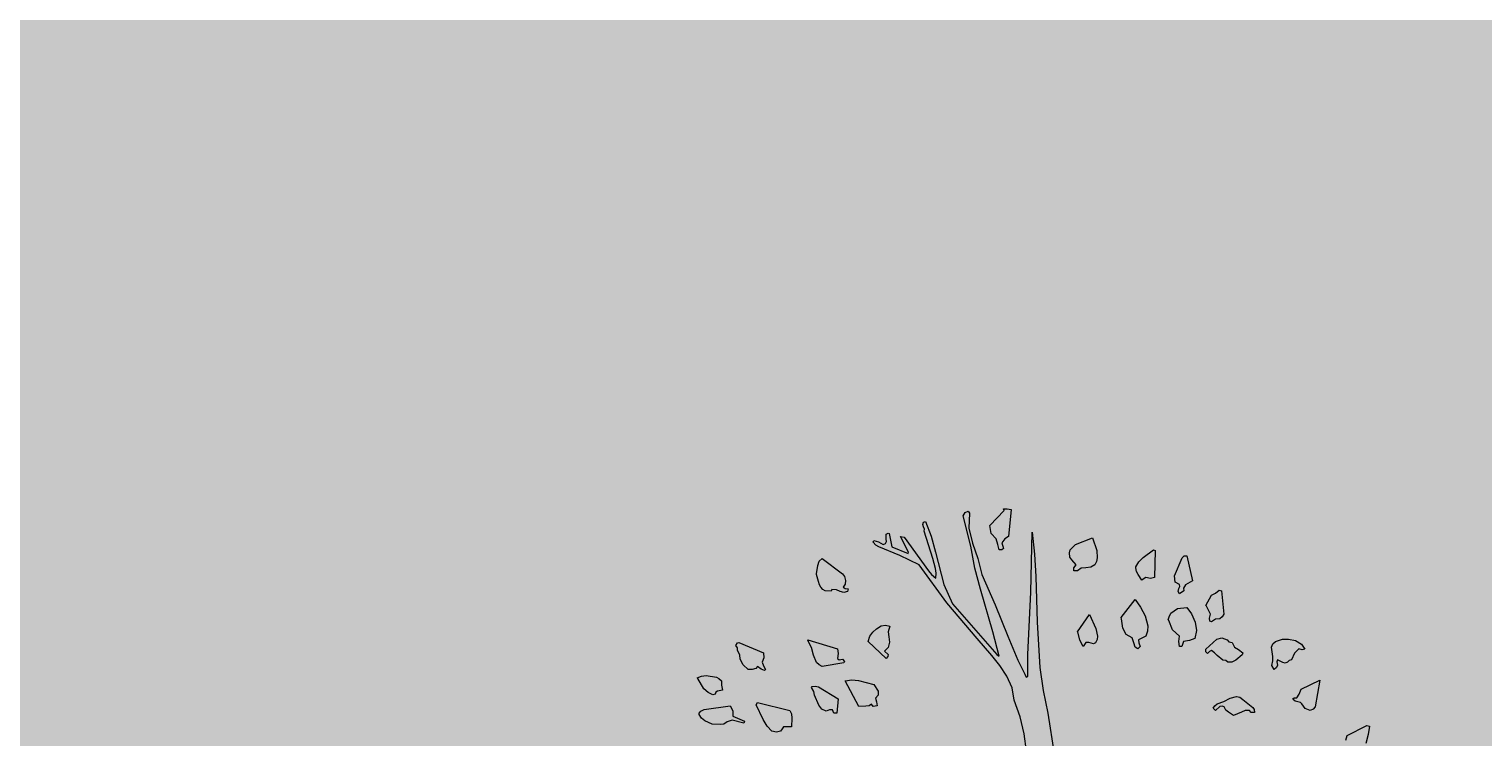
# Model space of a CAD drawing. Units: inches. Extents: x 84 to 1044, y -280 to 906.
# Tile 85 of 105: x 815 to 856, y 425 to 445. Entities that reach past the tile are written whole.
import ezdxf

# ---------------------------------------------------------------- set-up
doc = ezdxf.new("R2010")
doc.units = ezdxf.units.IN
doc.layers.add('A-ANNO-DIMS', color=2, linetype='Continuous', lineweight=18)
doc.layers.add('L-PLNT', color=114, linetype='Continuous', lineweight=15)
doc.layers.add('L-PLNT-PATT', color=9, linetype='Continuous', lineweight=9, true_color=0xafd9aa)
doc.styles.get("Standard").update_dxf_attribs({"font": 'arial.ttf'})
doc.dimstyles.get("Standard").update_dxf_attribs({"dimtxt": 0.18, "dimasz": 0.18, "dimexe": 0.18, "dimexo": 0.0625, "dimgap": 0.09, "dimtad": 0, "dimtih": 1, "dimtoh": 1, "dimdec": 4, "dimzin": 0, "dimdsep": 46, "dimtxsty": 'Standard', "dimcen": 0.09, "dimadec": 0, "dimazin": 0, "dimtfac": 1, "dimtdec": 4, "dimtofl": 0, "dimtmove": 0, "dimatfit": 3, "dimfxl": 1, "dimtolj": 1, "dimtzin": 0, "dimarcsym": 0})

# ---------------------------------------------------------------- blocks, each defined once
blk = doc.blocks.new('A$C37E508DF')
for p, q in [((0.6329, 1.5111), (0.6367, 1.5175)), ((0.6367, 1.5175), (0.6423, 1.5201)), ((0.6423, 1.5201), (0.6453, 1.5158)), ((0.6826, 1.493), (0.7096, 1.5209)), ((0.7083, 1.5239), (0.7152, 1.5244)), ((0.7096, 1.5209), (0.7083, 1.5239)), ((0.7152, 1.5244), (0.7225, 1.5231)), ((0.7225, 1.5231), (0.7174, 1.4729)), ((0.5583, 1.4948), (0.5596, 1.4995)), ((0.5596, 1.4905), (0.5583, 1.4948)), ((0.5596, 1.4995), (0.563, 1.5003)), ((0.5613, 1.4862), (0.5596, 1.4905)), ((0.563, 1.5003), (0.5737, 1.4733)), ((0.6475, 1.4545), (0.6329, 1.5111)), ((0.6453, 1.5158), (0.644, 1.4879)), ((0.6852, 1.4785), (0.6826, 1.493)), ((0.4657, 1.4622), (0.4669, 1.4652)), ((0.4708, 1.4566), (0.4657, 1.4622)), ((0.4669, 1.4652), (0.4755, 1.463)), ((0.4755, 1.463), (0.4845, 1.4575)), ((0.4884, 1.4596), (0.4905, 1.4635)), ((0.4897, 1.4772), (0.4935, 1.4789)), ((0.4897, 1.4678), (0.4897, 1.4772)), ((0.4905, 1.4635), (0.4897, 1.4678)), ((0.4935, 1.4789), (0.4952, 1.478)), ((0.4952, 1.478), (0.5004, 1.4532)), ((0.5313, 1.4437), (0.5167, 1.4729)), ((0.5167, 1.4729), (0.5231, 1.4716)), ((0.5231, 1.4716), (0.5686, 1.409)), ((0.5608, 1.4823), (0.5613, 1.4862)), ((0.5767, 1.4317), (0.5608, 1.4823)), ((0.5737, 1.4733), (0.5814, 1.4437)), ((0.644, 1.4879), (0.6505, 1.46)), ((0.6946, 1.4682), (0.6852, 1.4785)), ((0.6976, 1.4579), (0.6946, 1.4682)), ((0.7109, 1.4682), (0.7053, 1.4609)), ((0.7174, 1.4729), (0.7109, 1.4682)), ((0.7589, 1.3691), (0.7615, 1.481)), ((0.7615, 1.481), (0.7658, 1.4395)), ((0.8421, 1.4575), (0.8739, 1.4703)), ((0.8739, 1.4703), (0.882, 1.4463)), ((0.4764, 1.4532), (0.4708, 1.4566)), ((0.5154, 1.4373), (0.4764, 1.4532)), ((0.4845, 1.4575), (0.4884, 1.4596)), ((0.5004, 1.4532), (0.5308, 1.4412)), ((0.551, 1.4197), (0.5154, 1.4373)), ((0.5308, 1.4412), (0.5313, 1.4437)), ((0.5814, 1.4437), (0.5969, 1.3833)), ((0.6552, 1.4137), (0.6475, 1.4545)), ((0.6505, 1.46), (0.6603, 1.4317)), ((0.7002, 1.4476), (0.6976, 1.4579)), ((0.7049, 1.448), (0.7002, 1.4476)), ((0.7083, 1.4502), (0.7049, 1.448)), ((0.7053, 1.4609), (0.7083, 1.4502)), ((0.7658, 1.4395), (0.7684, 1.3979)), ((0.831, 1.4424), (0.8323, 1.4476)), ((0.8318, 1.4343), (0.831, 1.4424)), ((0.8323, 1.4476), (0.8357, 1.451)), ((0.8357, 1.451), (0.8421, 1.4575)), ((0.882, 1.4463), (0.8829, 1.433)), ((0.9686, 1.4334), (0.9875, 1.4476)), ((0.9875, 1.4476), (0.9905, 1.4467)), ((0.9905, 1.4467), (0.9896, 1.3966)), ((1.0411, 1.433), (1.045, 1.4365)), ((1.045, 1.4365), (1.0497, 1.4369)), ((1.0497, 1.4369), (1.0604, 1.3901)), ((0.3598, 1.403), (0.3628, 1.4189)), ((0.3628, 1.4189), (0.3649, 1.4266)), ((0.3649, 1.4266), (0.3709, 1.4317)), ((0.3709, 1.4317), (0.4086, 1.403)), ((0.6029, 1.3494), (0.551, 1.4197)), ((0.5686, 1.409), (0.5741, 1.4021)), ((0.5814, 1.4133), (0.5767, 1.4317)), ((0.5827, 1.4043), (0.5814, 1.4133)), ((0.6655, 1.3743), (0.6552, 1.4137)), ((0.6603, 1.4317), (0.668, 1.4021)), ((0.8353, 1.4292), (0.8318, 1.4343)), ((0.8434, 1.4197), (0.8353, 1.4292)), ((0.8391, 1.4141), (0.8434, 1.4197)), ((0.8395, 1.4086), (0.8391, 1.4141)), ((0.846, 1.4086), (0.8395, 1.4086)), ((0.8528, 1.4137), (0.846, 1.4086)), ((0.8619, 1.4146), (0.8528, 1.4137)), ((0.8709, 1.4154), (0.8619, 1.4146)), ((0.8781, 1.4197), (0.8709, 1.4154)), ((0.8816, 1.4262), (0.8781, 1.4197)), ((0.8829, 1.433), (0.8816, 1.4262)), ((0.9545, 1.4159), (0.9605, 1.4257)), ((0.9549, 1.4146), (0.9545, 1.4159)), ((0.9558, 1.4077), (0.9549, 1.4146)), ((0.9605, 1.4257), (0.9686, 1.4334)), ((1.0269, 1.3996), (1.0411, 1.433)), ((0.3602, 1.4021), (0.3598, 1.403)), ((0.364, 1.3888), (0.3602, 1.4021)), ((0.3657, 1.3828), (0.364, 1.3888)), ((0.3683, 1.3781), (0.3657, 1.3828)), ((0.4086, 1.403), (0.4125, 1.3979)), ((0.4134, 1.3837), (0.4099, 1.3781)), ((0.4125, 1.3979), (0.4142, 1.391)), ((0.4142, 1.391), (0.4134, 1.3837)), ((0.5741, 1.4021), (0.5823, 1.3953)), ((0.5823, 1.3953), (0.5827, 1.4043)), ((0.5969, 1.3833), (0.6132, 1.3472)), ((0.668, 1.4021), (0.6925, 1.3455)), ((0.7684, 1.3979), (0.771, 1.3134)), ((0.9592, 1.4017), (0.9558, 1.4077)), ((0.966, 1.3914), (0.9592, 1.4017)), ((0.9703, 1.3944), (0.966, 1.3914)), ((0.9733, 1.3966), (0.9703, 1.3944)), ((0.9819, 1.3944), (0.9733, 1.3966)), ((0.9896, 1.3966), (0.9819, 1.3944)), ((1.0282, 1.3876), (1.0269, 1.3996)), ((1.0359, 1.3833), (1.0282, 1.3876)), ((1.0368, 1.3794), (1.0359, 1.3833)), ((1.0471, 1.3824), (1.0432, 1.3764)), ((1.0604, 1.3901), (1.0471, 1.3824)), ((0.3718, 1.3738), (0.3683, 1.3781)), ((0.3765, 1.3713), (0.3718, 1.3738)), ((0.3872, 1.3708), (0.3765, 1.3713)), ((0.3885, 1.3738), (0.3872, 1.3708)), ((0.3971, 1.3734), (0.3885, 1.3738)), ((0.4039, 1.3704), (0.3971, 1.3734)), ((0.4108, 1.3683), (0.4039, 1.3704)), ((0.4099, 1.3781), (0.4134, 1.376)), ((0.4176, 1.37), (0.4108, 1.3683)), ((0.4134, 1.376), (0.4189, 1.3751)), ((0.4189, 1.3751), (0.4176, 1.37)), ((0.6882, 1.2949), (0.6655, 1.3743)), ((0.7538, 1.2529), (0.7589, 1.3691)), ((0.9274, 1.3215), (0.9532, 1.3554)), ((0.9532, 1.3554), (0.9635, 1.3413)), ((1.0334, 1.37), (1.0351, 1.376)), ((1.0359, 1.3661), (1.0334, 1.37)), ((1.0351, 1.376), (1.0368, 1.3794)), ((1.0441, 1.3717), (1.0359, 1.3661)), ((1.0432, 1.3764), (1.0441, 1.3717)), ((1.0848, 1.3443), (1.0955, 1.3631)), ((1.0955, 1.3631), (1.1033, 1.367)), ((1.1033, 1.367), (1.1097, 1.373)), ((1.1097, 1.373), (1.114, 1.3717)), ((1.114, 1.3717), (1.1183, 1.328)), ((0.6595, 1.2829), (0.6029, 1.3494)), ((0.6132, 1.3472), (0.6959, 1.2529)), ((0.6925, 1.3455), (0.7161, 1.2868)), ((0.846, 1.2949), (0.8687, 1.3271)), ((0.8687, 1.3271), (0.8803, 1.3014)), ((0.9635, 1.3413), (0.9721, 1.325)), ((1.0171, 1.3232), (1.0197, 1.3297)), ((1.0197, 1.3297), (1.0321, 1.3387)), ((1.0321, 1.3387), (1.0497, 1.3404)), ((1.0497, 1.3404), (1.0587, 1.3284)), ((1.0587, 1.3284), (1.0651, 1.3134)), ((1.0861, 1.343), (1.0848, 1.3443)), ((1.0938, 1.328), (1.0861, 1.343)), ((1.0917, 1.3207), (1.0938, 1.328)), ((1.1183, 1.328), (1.1153, 1.3228)), ((0.4648, 1.2945), (0.4717, 1.3009)), ((0.4717, 1.3009), (0.4807, 1.3065)), ((0.4807, 1.3065), (0.4884, 1.3074)), ((0.4884, 1.3074), (0.4965, 1.3057)), ((0.4965, 1.3057), (0.4935, 1.2954)), ((0.771, 1.3134), (0.7761, 1.2285)), ((0.8803, 1.3014), (0.8833, 1.2872)), ((0.9279, 1.3194), (0.9274, 1.3215)), ((0.9305, 1.3018), (0.9279, 1.3194)), ((0.9365, 1.2902), (0.9305, 1.3018)), ((0.9721, 1.325), (0.9768, 1.3061)), ((0.9768, 1.3061), (0.9763, 1.2962)), ((1.0149, 1.3172), (1.0171, 1.3232)), ((1.0162, 1.3164), (1.0149, 1.3172)), ((1.0231, 1.2988), (1.0162, 1.3164)), ((1.0651, 1.3134), (1.0677, 1.2975)), ((1.0925, 1.3151), (1.0917, 1.3207)), ((1.0955, 1.3138), (1.0925, 1.3151)), ((1.1028, 1.3185), (1.0955, 1.3138)), ((1.111, 1.3194), (1.1028, 1.3185)), ((1.1153, 1.3228), (1.111, 1.3194)), ((0.2101, 1.2696), (0.2127, 1.2744)), ((0.2127, 1.2744), (0.2152, 1.2752)), ((0.2152, 1.2752), (0.2611, 1.2559)), ((0.3439, 1.2804), (0.3992, 1.2636)), ((0.3439, 1.2787), (0.3439, 1.2804)), ((0.3507, 1.2662), (0.3439, 1.2787)), ((0.4562, 1.2774), (0.4597, 1.2868)), ((0.4897, 1.2452), (0.4562, 1.2774)), ((0.4597, 1.2868), (0.4648, 1.2945)), ((0.4935, 1.2954), (0.4948, 1.2855)), ((0.4961, 1.2756), (0.4935, 1.2658)), ((0.4948, 1.2855), (0.4961, 1.2756)), ((0.6865, 1.2508), (0.6595, 1.2829)), ((0.7002, 1.2495), (0.6882, 1.2949)), ((0.7161, 1.2868), (0.7349, 1.2422)), ((0.8473, 1.2924), (0.846, 1.2949)), ((0.8507, 1.2795), (0.8473, 1.2924)), ((0.8567, 1.2679), (0.8507, 1.2795)), ((0.8619, 1.2752), (0.8567, 1.2679)), ((0.867, 1.2752), (0.8619, 1.2752)), ((0.8713, 1.2739), (0.867, 1.2752)), ((0.8756, 1.2726), (0.8713, 1.2739)), ((0.8799, 1.2744), (0.8756, 1.2726)), ((0.8829, 1.2808), (0.8799, 1.2744)), ((0.8833, 1.2872), (0.8829, 1.2808)), ((0.9476, 1.2842), (0.9365, 1.2902)), ((0.951, 1.2748), (0.9476, 1.2842)), ((0.9532, 1.2666), (0.951, 1.2748)), ((0.9733, 1.2868), (0.9596, 1.2799)), ((0.9596, 1.2799), (0.9605, 1.2744)), ((0.9605, 1.2744), (0.9626, 1.2679)), ((0.9763, 1.2962), (0.9733, 1.2868)), ((1.0359, 1.2868), (1.0231, 1.2988)), ((1.0347, 1.2769), (1.0359, 1.2868)), ((1.0359, 1.2679), (1.0347, 1.2769)), ((1.0432, 1.2774), (1.0402, 1.2679)), ((1.0544, 1.2791), (1.0432, 1.2774)), ((1.0647, 1.2829), (1.0544, 1.2791)), ((1.0677, 1.2975), (1.0647, 1.2829)), ((1.0848, 1.2628), (1.1054, 1.2817)), ((1.1054, 1.2817), (1.1148, 1.2842)), ((1.1148, 1.2842), (1.1247, 1.2804)), ((1.1247, 1.2804), (1.1281, 1.2765)), ((1.1281, 1.2765), (1.1341, 1.2752)), ((1.1341, 1.2752), (1.1384, 1.2666)), ((1.2075, 1.2666), (1.21, 1.2726)), ((1.21, 1.2726), (1.2147, 1.2774)), ((1.2147, 1.2774), (1.2276, 1.2817)), ((1.2276, 1.2817), (1.2392, 1.2817)), ((1.2392, 1.2817), (1.2521, 1.2787)), ((1.2521, 1.2787), (1.2632, 1.2722)), ((0.2127, 1.2654), (0.2101, 1.2696)), ((0.2127, 1.2602), (0.2127, 1.2654)), ((0.2174, 1.2521), (0.2127, 1.2602)), ((0.2182, 1.2443), (0.2174, 1.2521)), ((0.262, 1.2465), (0.2586, 1.2388)), ((0.2611, 1.2559), (0.262, 1.2465)), ((0.3546, 1.2516), (0.3507, 1.2662)), ((0.3602, 1.2383), (0.3546, 1.2516)), ((0.3992, 1.2636), (0.4005, 1.2546)), ((0.4005, 1.2546), (0.3992, 1.2452)), ((0.4935, 1.2658), (0.4867, 1.2589)), ((0.4867, 1.2589), (0.4935, 1.2529)), ((0.4931, 1.2491), (0.4897, 1.2452)), ((0.4935, 1.2529), (0.4931, 1.2491)), ((0.7015, 1.2323), (0.6865, 1.2508)), ((0.6959, 1.2529), (0.7002, 1.2495)), ((0.7538, 1.2122), (0.7538, 1.2529)), ((0.9583, 1.2636), (0.9532, 1.2666)), ((0.9626, 1.2679), (0.9583, 1.2636)), ((1.0402, 1.2679), (1.0359, 1.2679)), ((1.0852, 1.2576), (1.0848, 1.2628)), ((1.0883, 1.2546), (1.0852, 1.2576)), ((1.0921, 1.2585), (1.0883, 1.2546)), ((1.0955, 1.2602), (1.0921, 1.2585)), ((1.1015, 1.2559), (1.0955, 1.2602)), ((1.1063, 1.2508), (1.1015, 1.2559)), ((1.117, 1.2422), (1.1063, 1.2508)), ((1.1384, 1.2666), (1.1461, 1.2619)), ((1.1526, 1.2521), (1.141, 1.2422)), ((1.1461, 1.2619), (1.1539, 1.2559)), ((1.1539, 1.2559), (1.1526, 1.2521)), ((1.2096, 1.2491), (1.2075, 1.2666)), ((1.21, 1.2409), (1.2096, 1.2491)), ((1.2503, 1.2551), (1.2448, 1.2431)), ((1.2585, 1.2636), (1.2503, 1.2551)), ((1.2645, 1.2615), (1.2585, 1.2636)), ((1.2632, 1.2722), (1.2692, 1.2628)), ((1.2692, 1.2628), (1.2645, 1.2615)), ((0.2234, 1.2336), (0.2182, 1.2443)), ((0.2328, 1.2251), (0.2234, 1.2336)), ((0.2401, 1.2251), (0.2328, 1.2251)), ((0.2474, 1.2268), (0.2401, 1.2251)), ((0.2504, 1.2306), (0.2474, 1.2268)), ((0.2568, 1.2255), (0.2504, 1.2306)), ((0.2633, 1.2229), (0.2568, 1.2255)), ((0.2586, 1.2388), (0.2611, 1.2319)), ((0.2611, 1.2319), (0.265, 1.2251)), ((0.265, 1.2251), (0.2633, 1.2229)), ((0.3649, 1.2336), (0.3602, 1.2383)), ((0.3709, 1.2306), (0.3649, 1.2336)), ((0.4112, 1.2375), (0.3709, 1.2306)), ((0.3992, 1.2452), (0.4026, 1.2431)), ((0.4026, 1.2431), (0.4086, 1.2443)), ((0.4086, 1.2443), (0.4121, 1.2401)), ((0.4121, 1.2401), (0.4112, 1.2375)), ((0.7148, 1.2126), (0.7015, 1.2323)), ((0.7349, 1.2422), (0.7482, 1.216)), ((0.7761, 1.2285), (0.7821, 1.1856)), ((1.1221, 1.2418), (1.117, 1.2422)), ((1.126, 1.2388), (1.1221, 1.2418)), ((1.1337, 1.2388), (1.126, 1.2388)), ((1.141, 1.2422), (1.1337, 1.2388)), ((1.2079, 1.2323), (1.21, 1.2409)), ((1.2126, 1.2251), (1.2079, 1.2323)), ((1.2169, 1.2285), (1.2126, 1.2251)), ((1.2186, 1.2332), (1.2169, 1.2285)), ((1.2186, 1.2431), (1.2173, 1.2392)), ((1.2173, 1.2392), (1.2186, 1.2332)), ((1.2285, 1.2383), (1.2186, 1.2431)), ((1.2328, 1.2366), (1.2285, 1.2383)), ((1.2371, 1.2388), (1.2328, 1.2366)), ((1.2405, 1.2418), (1.2371, 1.2388)), ((1.2448, 1.2431), (1.2405, 1.2418)), ((0.1376, 1.2092), (0.1458, 1.2126)), ((0.1389, 1.2079), (0.1376, 1.2092)), ((0.1505, 1.189), (0.1389, 1.2079)), ((0.1458, 1.2126), (0.1548, 1.2135)), ((0.1548, 1.2135), (0.1741, 1.2109)), ((0.1741, 1.2109), (0.1784, 1.2083)), ((0.1784, 1.2083), (0.1831, 1.204)), ((0.1831, 1.204), (0.1831, 1.1959)), ((0.1831, 1.1959), (0.1848, 1.1865)), ((0.3507, 1.1916), (0.352, 1.1933)), ((0.355, 1.1839), (0.3507, 1.1916)), ((0.352, 1.1933), (0.3576, 1.1942)), ((0.3576, 1.1942), (0.364, 1.1929)), ((0.364, 1.1929), (0.4005, 1.1702)), ((0.4134, 1.204), (0.4258, 1.2058)), ((0.4391, 1.156), (0.4134, 1.204)), ((0.4258, 1.2058), (0.4382, 1.2045)), ((0.4382, 1.2045), (0.4669, 1.1972)), ((0.4669, 1.1972), (0.4747, 1.1843)), ((0.7246, 1.1908), (0.7148, 1.2126)), ((0.7482, 1.216), (0.7508, 1.2109)), ((0.7508, 1.2109), (0.7538, 1.2122)), ((1.2628, 1.1882), (1.2975, 1.2053)), ((1.2975, 1.2053), (1.2885, 1.1556)), ((0.1582, 1.1822), (0.1505, 1.189)), ((0.1668, 1.1775), (0.1582, 1.1822)), ((0.1711, 1.1792), (0.1668, 1.1775)), ((0.1728, 1.1826), (0.1711, 1.1792)), ((0.1758, 1.1847), (0.1728, 1.1826)), ((0.1788, 1.1852), (0.1758, 1.1847)), ((0.1848, 1.1865), (0.1788, 1.1852)), ((0.3563, 1.177), (0.355, 1.1839)), ((0.3645, 1.1586), (0.3563, 1.177)), ((0.4005, 1.1702), (0.3979, 1.1436)), ((0.4751, 1.177), (0.47, 1.1714)), ((0.47, 1.1714), (0.4721, 1.1646)), ((0.4721, 1.1646), (0.473, 1.1573)), ((0.4747, 1.1843), (0.4751, 1.177)), ((0.7281, 1.168), (0.7246, 1.1908)), ((0.7396, 1.1371), (0.7281, 1.168)), ((0.7821, 1.1856), (0.7911, 1.1436)), ((1.1063, 1.1612), (1.1187, 1.1655)), ((1.1187, 1.1655), (1.1307, 1.1714)), ((1.1307, 1.1714), (1.1423, 1.1744)), ((1.1423, 1.1744), (1.1483, 1.1732)), ((1.1483, 1.1732), (1.1539, 1.1693)), ((1.1539, 1.1693), (1.1727, 1.1543)), ((1.2469, 1.1702), (1.2495, 1.1723)), ((1.2478, 1.1693), (1.2469, 1.1702)), ((1.2516, 1.1659), (1.2478, 1.1693)), ((1.2495, 1.1723), (1.2546, 1.1719)), ((1.2563, 1.1646), (1.2516, 1.1659)), ((1.2546, 1.1719), (1.2589, 1.1792)), ((1.2611, 1.1637), (1.2563, 1.1646)), ((1.2589, 1.1792), (1.2628, 1.1882)), ((0.1419, 1.1436), (0.1449, 1.1474)), ((0.1419, 1.141), (0.1419, 1.1436)), ((0.1462, 1.1342), (0.1419, 1.141)), ((0.1449, 1.1474), (0.1509, 1.1504)), ((0.1509, 1.1504), (0.1994, 1.1573)), ((0.1994, 1.1573), (0.2041, 1.1479)), ((0.2041, 1.1479), (0.2045, 1.138)), ((0.2045, 1.138), (0.226, 1.129)), ((0.2478, 1.1594), (0.2504, 1.1637)), ((0.2607, 1.1316), (0.2478, 1.1594)), ((0.2504, 1.1637), (0.3104, 1.1487)), ((0.3104, 1.1487), (0.3134, 1.1423)), ((0.3134, 1.1423), (0.3139, 1.1346)), ((0.37, 1.1509), (0.3645, 1.1586)), ((0.3778, 1.1474), (0.37, 1.1509)), ((0.3842, 1.15), (0.3778, 1.1474)), ((0.3898, 1.15), (0.3842, 1.15)), ((0.3923, 1.1436), (0.3898, 1.15)), ((0.3979, 1.1436), (0.3923, 1.1436)), ((0.4519, 1.1564), (0.4391, 1.156)), ((0.458, 1.1573), (0.4519, 1.1564)), ((0.4622, 1.1607), (0.458, 1.1573)), ((0.4657, 1.156), (0.4622, 1.1607)), ((0.473, 1.1573), (0.4657, 1.156)), ((0.7469, 1.1054), (0.7396, 1.1371)), ((0.7911, 1.1436), (0.8027, 1.0677)), ((1.099, 1.153), (1.102, 1.1573)), ((1.1033, 1.1487), (1.099, 1.153)), ((1.102, 1.1573), (1.1063, 1.1612)), ((1.111, 1.156), (1.1033, 1.1487)), ((1.1153, 1.1564), (1.111, 1.156)), ((1.1191, 1.1556), (1.1153, 1.1564)), ((1.1226, 1.1492), (1.1191, 1.1556)), ((1.1273, 1.1453), (1.1226, 1.1492)), ((1.1367, 1.1393), (1.1273, 1.1453)), ((1.1517, 1.1453), (1.1367, 1.1393)), ((1.1586, 1.1483), (1.1517, 1.1453)), ((1.1663, 1.1487), (1.1586, 1.1483)), ((1.1697, 1.1449), (1.1663, 1.1487)), ((1.1757, 1.1449), (1.1697, 1.1449)), ((1.1727, 1.1543), (1.1749, 1.1504)), ((1.1749, 1.1504), (1.1757, 1.1449)), ((1.2641, 1.1612), (1.2611, 1.1637)), ((1.2701, 1.1522), (1.2641, 1.1612)), ((1.2791, 1.1487), (1.2701, 1.1522)), ((1.2851, 1.1509), (1.2791, 1.1487)), ((1.2885, 1.1556), (1.2851, 1.1509)), ((0.1522, 1.1294), (0.1462, 1.1342)), ((0.1655, 1.1234), (0.1522, 1.1294)), ((0.181, 1.1226), (0.1655, 1.1234)), ((0.1878, 1.1234), (0.181, 1.1226)), ((0.1938, 1.1273), (0.1878, 1.1234)), ((0.2032, 1.1303), (0.1938, 1.1273)), ((0.2247, 1.1251), (0.2032, 1.1303)), ((0.226, 1.129), (0.2247, 1.1251)), ((0.268, 1.1196), (0.2607, 1.1316)), ((0.277, 1.1101), (0.268, 1.1196)), ((0.2856, 1.108), (0.277, 1.1101)), ((0.2933, 1.1101), (0.2856, 1.108)), ((0.2959, 1.1144), (0.2933, 1.1101)), ((0.2984, 1.1179), (0.2959, 1.1144)), ((0.3066, 1.1179), (0.2984, 1.1179)), ((0.3134, 1.1183), (0.3066, 1.1179)), ((0.3139, 1.1346), (0.3134, 1.1183)), ((1.3485, 1.102), (1.385, 1.1209)), ((1.385, 1.1209), (1.3897, 1.1196)), ((1.3897, 1.1196), (1.3875, 1.1037)), ((0.7512, 1.0728), (0.7469, 1.1054)), ((1.3455, 1.0934), (1.3485, 1.102)), ((1.3875, 1.1037), (1.3828, 1.087))]:
    blk.add_line(p, q)
blk = doc.blocks.new('*D62')
at = {"layer": 'A-ANNO-DIMS', "color": 0, "lineweight": -2, "transparency": 16777216}
for p, q in [((203.179, 709.183), (203.179, 905.9)), ((896.074, 400.183), (896.074, 905.9)), ((203.359, 905.72), (549.232, 905.72)), ((895.894, 905.72), (550.021, 905.72))]:
    blk.add_line(p, q, dxfattribs=at)
at = {"layer": 'A-ANNO-DIMS', "color": 0, "transparency": 16777216}
for points in [[(203.359, 905.75), (203.359, 905.69), (203.179, 905.72)], [(895.894, 905.75), (895.894, 905.69), (896.074, 905.72)]]:
    blk.add_solid(points, dxfattribs=at)
at = {"layer": 'Defpoints', "color": 0, "transparency": 16777216}
for p in [(896.074, 905.72), (203.179, 709.12), (896.074, 400.12)]:
    blk.add_point(p, dxfattribs=at)
at = {"layer": 'A-ANNO-DIMS', "color": 0, "transparency": 16777216, "insert": (549.627, 905.72), "char_height": 0.18, "attachment_point": 5}
blk.add_mtext('\\A1;692.9', dxfattribs=at)
blk = doc.blocks.new('*D63')
at = {"layer": 'A-ANNO-DIMS', "color": 0, "lineweight": -2, "transparency": 16777216}
for p, q in [((833.136, 709.12), (1043.768, 709.12)), ((1043.588, 708.94), (1043.588, 400.302)), ((1043.588, 91.3), (1043.588, 399.938)), ((896.136, 91.12), (1043.768, 91.12))]:
    blk.add_line(p, q, dxfattribs=at)
at = {"layer": 'A-ANNO-DIMS', "color": 0, "transparency": 16777216}
for points in [[(1043.558, 708.94), (1043.618, 708.94), (1043.588, 709.12)], [(1043.558, 91.3), (1043.618, 91.3), (1043.588, 91.12)]]:
    blk.add_solid(points, dxfattribs=at)
at = {"layer": 'Defpoints', "color": 0, "transparency": 16777216}
for p in [(833.074, 709.12), (1043.588, 709.12), (896.074, 91.12)]:
    blk.add_point(p, dxfattribs=at)
at = {"layer": 'A-ANNO-DIMS', "color": 0, "transparency": 16777216, "insert": (1043.588, 400.12), "char_height": 0.18, "attachment_point": 5}
blk.add_mtext('\\A1;618', dxfattribs=at)

msp = doc.modelspace()

# ---------------------------------------------------------------- hatches: boundary and pattern name
at = {"layer": 'L-PLNT-PATT', "transparency": 33554597}
h = msp.add_hatch(color=256, dxfattribs=at)
h.dxf.hatch_style = 1
h.paths.add_polyline_path([(896.074, 511.12), (704.074, 511.12), (704.074, 491.62), (704.074, 419.62), (704.074, 400.12), (833.074, 400.12), (896.074, 400.12)])

# ---------------------------------------------------------------- block references
at = {"layer": 'L-PLNT', "xscale": 15.19586232982809, "yscale": 15.19586232982809, "zscale": 15.19586232982809}
msp.add_blockref('A$C37E508DF', (831.605, 408.742), dxfattribs=at)

# ---------------------------------------------------------------- dimensions: what is measured, and where the dimension line sits
at = {"layer": 'A-ANNO-DIMS'}
dim = msp.add_linear_dim(base=(896.074, 905.72), p1=(203.179, 709.12), p2=(896.074, 400.12), dimstyle='Standard', override={"dimdec": 1, "dimlfac": 1, "dimrnd": 0, "dimzin": 0, "dimdsep": 46, "dimlunit": 2}, dxfattribs=at)
dim.commit()
dim.dimension.update_dxf_attribs({"geometry": '*D62', "text_midpoint": (549.627, 905.72)})
dim = msp.add_linear_dim(base=(1043.588, 709.12), p1=(896.074, 91.12), p2=(833.074, 709.12), angle=90, dimstyle='Standard', override={"dimdec": 0, "dimlfac": 1, "dimrnd": 0, "dimzin": 0, "dimdsep": 46, "dimlunit": 2}, dxfattribs=at)
dim.commit()
dim.dimension.update_dxf_attribs({"geometry": '*D63', "text_midpoint": (1043.588, 400.12)})

doc.saveas('drawing.dxf')
